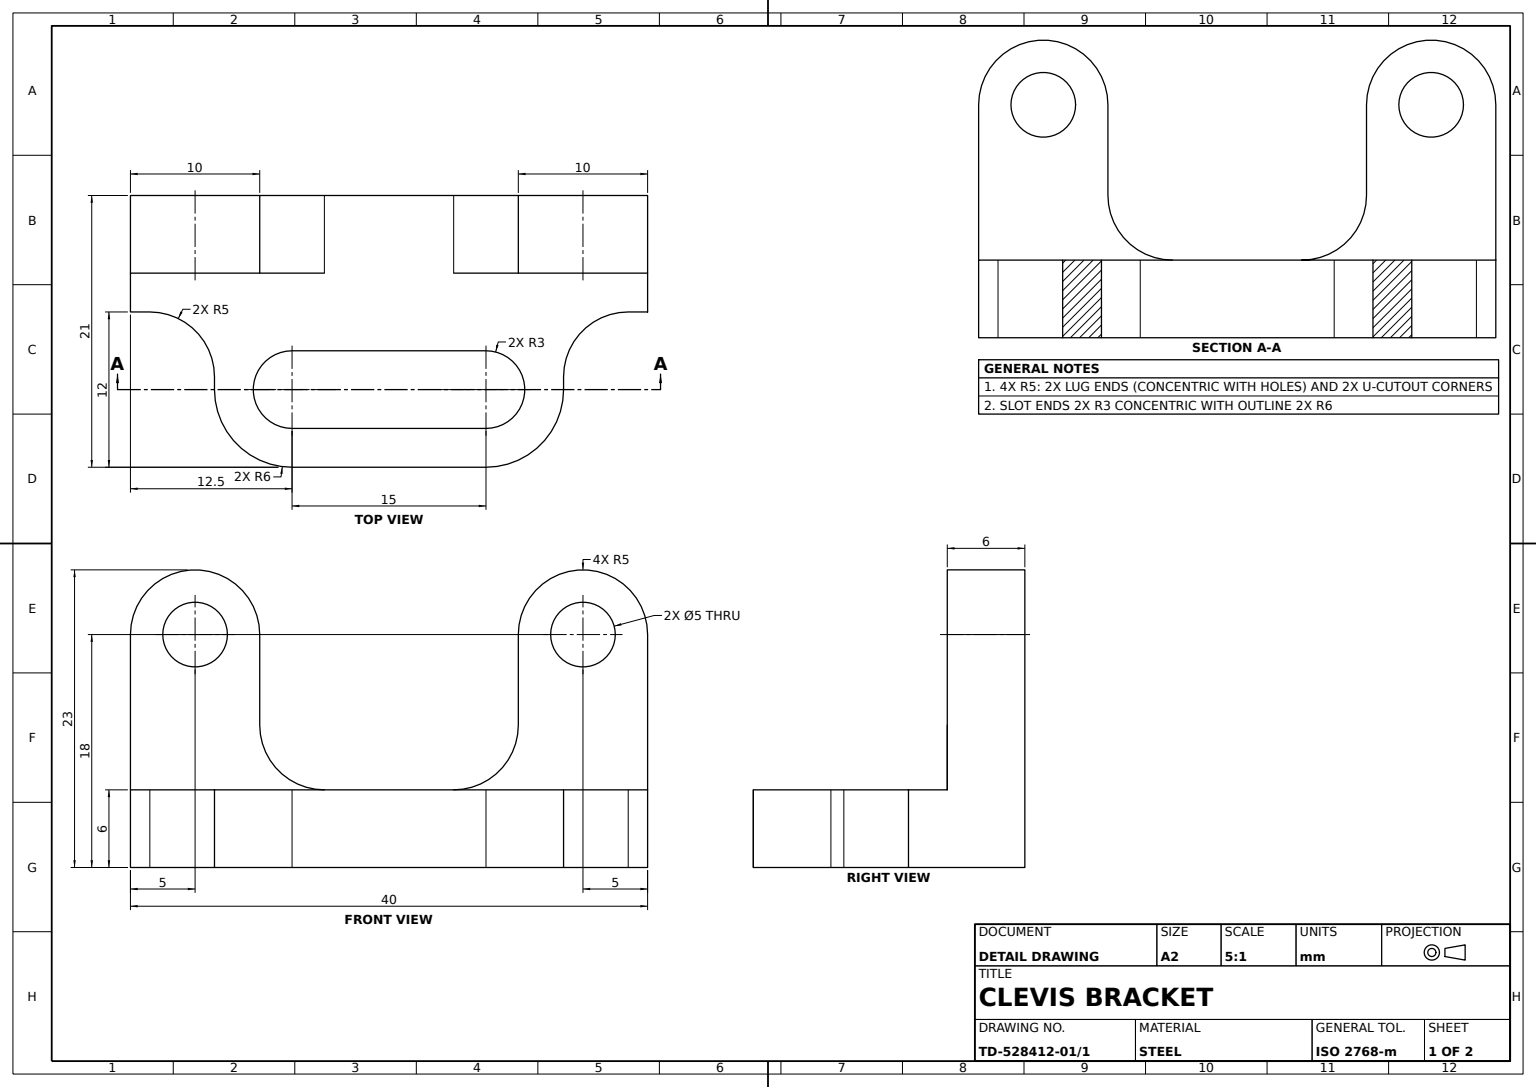
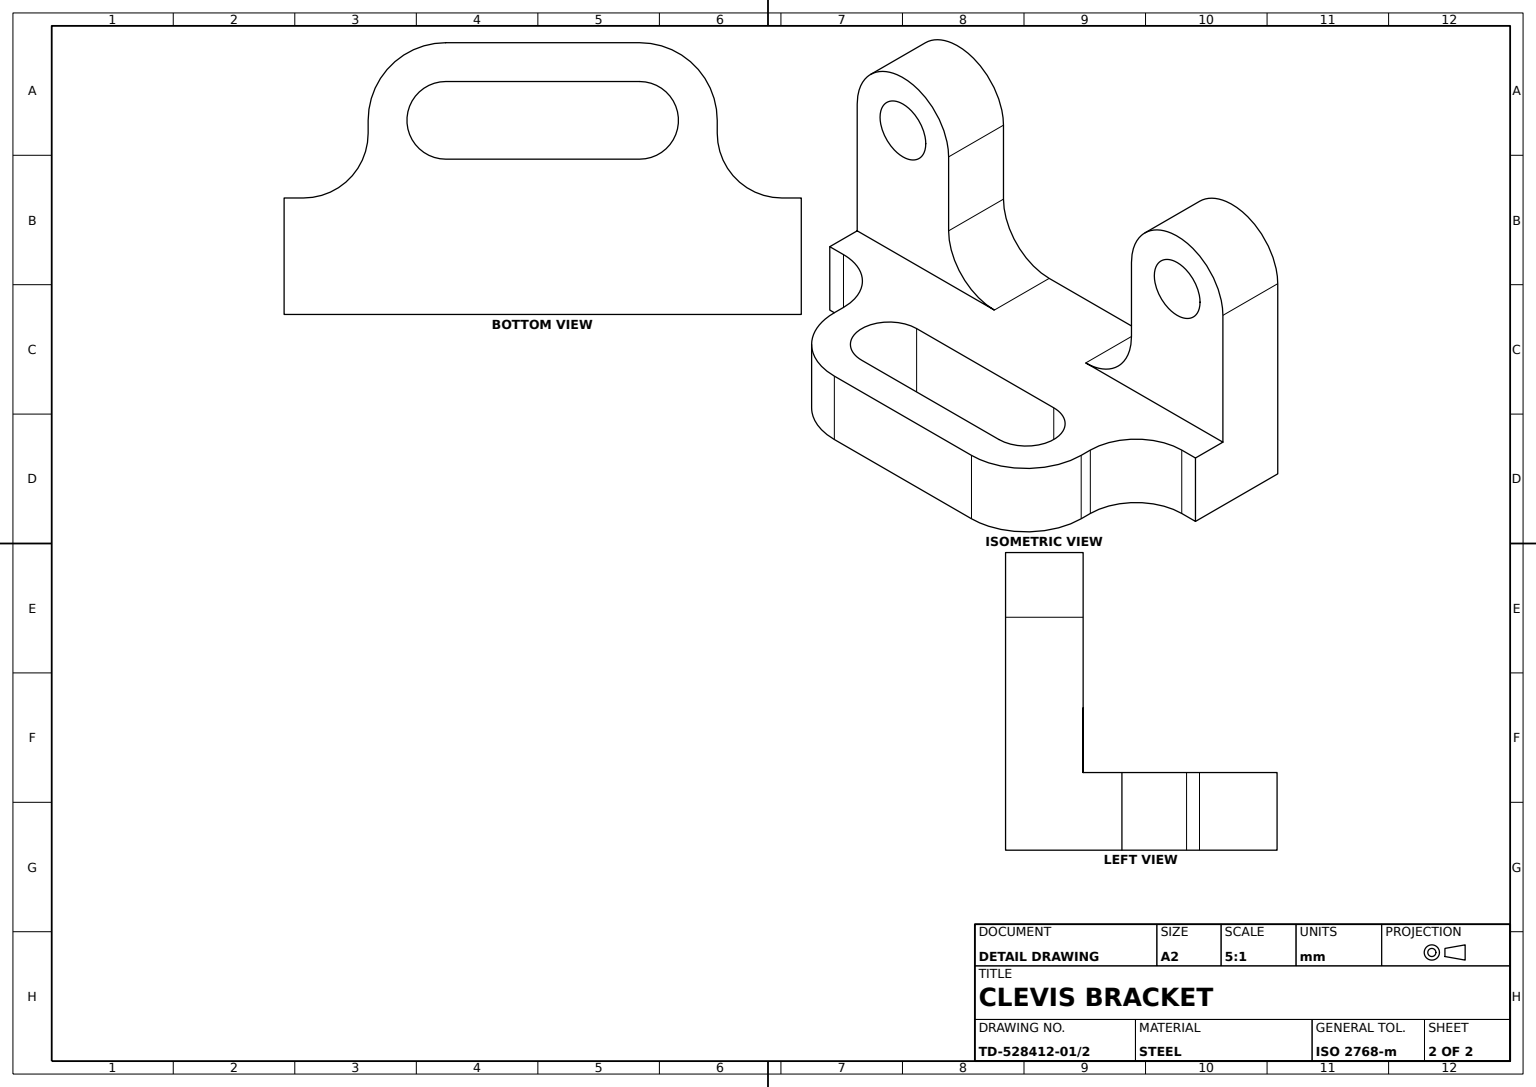
from build123d import *

# Parameters (mm, degrees)
BASE_PLATE_DEPTH        = 3
CLEVIS_LUGS_PROFILE_W   = 40
CLEVIS_LUGS_PROFILE_H   = 6
CLEVIS_LUGS_PROFILE_R   = 5
CLEVIS_LUGS_PROFILE_R_2 = 2.5
CLEVIS_LUGS_DEPTH       = 3


with BuildPart() as part:
    # Base Plate Profile → Base Plate (new, symmetric)
    with BuildSketch(Plane(origin=(0, 0, 0), x_dir=(1, 0, 0), z_dir=(0, 1, 0))):
        with BuildLine():
            Line((-20, 0), (20, 0))
            Line((20, 0), (20, -6))
            Line((20, -6), (18.5, -6))
            ThreePointArc((18.5, -6), (14.964466094, -7.464466094), (13.5, -11))
            Line((13.5, -11), (13.5, -12))
            ThreePointArc((13.5, -12), (11.742640687, -16.242640687), (7.5, -18))
            Line((7.5, -18), (-7.5, -18))
            ThreePointArc((-7.5, -18), (-11.742640687, -16.242640687), (-13.5, -12))
            Line((-13.5, -12), (-13.5, -11))
            ThreePointArc((-13.5, -11), (-14.964466094, -7.464466094), (-18.5, -6))
            Line((-18.5, -6), (-20, -6))
            Line((-20, -6), (-20, 0))
        make_face()
        with BuildLine():
            Line((-7.5, -9), (7.5, -9))
            ThreePointArc((7.5, -9), (10.5, -12), (7.5, -15))
            Line((7.5, -15), (-7.5, -15))
            ThreePointArc((-7.5, -15), (-10.5, -12), (-7.5, -9))
        make_face(mode=Mode.SUBTRACT)
    extrude(amount=BASE_PLATE_DEPTH, both=True)

    # Clevis Lugs Profile → Clevis Lugs (add, symmetric)
    # profile 1 of 5: a face of its own
    with BuildSketch(Plane(origin=(0, 0, 0), x_dir=(-1, 0, 0), z_dir=(0, 0, -1))):
        Rectangle(CLEVIS_LUGS_PROFILE_W, CLEVIS_LUGS_PROFILE_H)
    # profile 2 of 5: a face of its own
    with BuildSketch(Plane(origin=(0, 0, 0), x_dir=(-1, 0, 0), z_dir=(0, 0, -1))):
        with BuildLine():
            Line((-20, 15), (-20, 3))
            Line((-20, 3), (-5, 3))
            ThreePointArc((-5, 3), (-8.535533906, 4.464466094), (-10, 8))
            Line((-10, 8), (-10, 15))
            ThreePointArc((-10, 15), (-15, 10), (-20, 15))
        make_face()
    # profile 3 of 5: a face of its own
    with BuildSketch(Plane(origin=(0, 0, 0), x_dir=(-1, 0, 0), z_dir=(0, 0, -1))):
        with BuildLine():
            Line((5, 3), (20, 3))
            Line((20, 3), (20, 15))
            ThreePointArc((20, 15), (15, 10), (10, 15))
            Line((10, 15), (10, 8))
            ThreePointArc((10, 8), (8.535533906, 4.464466094), (5, 3))
        make_face()
    # profile 4 of 5: a face of its own
    with BuildSketch(Plane(origin=(0, 0, 0), x_dir=(-1, 0, 0), z_dir=(0, 0, -1))):
        with Locations((15, 15)):
            Circle(CLEVIS_LUGS_PROFILE_R)
        with Locations((15, 15)):
            Circle(CLEVIS_LUGS_PROFILE_R_2, mode=Mode.SUBTRACT)
    # profile 5 of 5: a face of its own
    with BuildSketch(Plane(origin=(0, 0, 0), x_dir=(-1, 0, 0), z_dir=(0, 0, -1))):
        with Locations((-15, 15)):
            Circle(CLEVIS_LUGS_PROFILE_R)
        with Locations((-15, 15)):
            Circle(CLEVIS_LUGS_PROFILE_R_2, mode=Mode.SUBTRACT)
    extrude(amount=CLEVIS_LUGS_DEPTH, both=True)


solid = part.part
